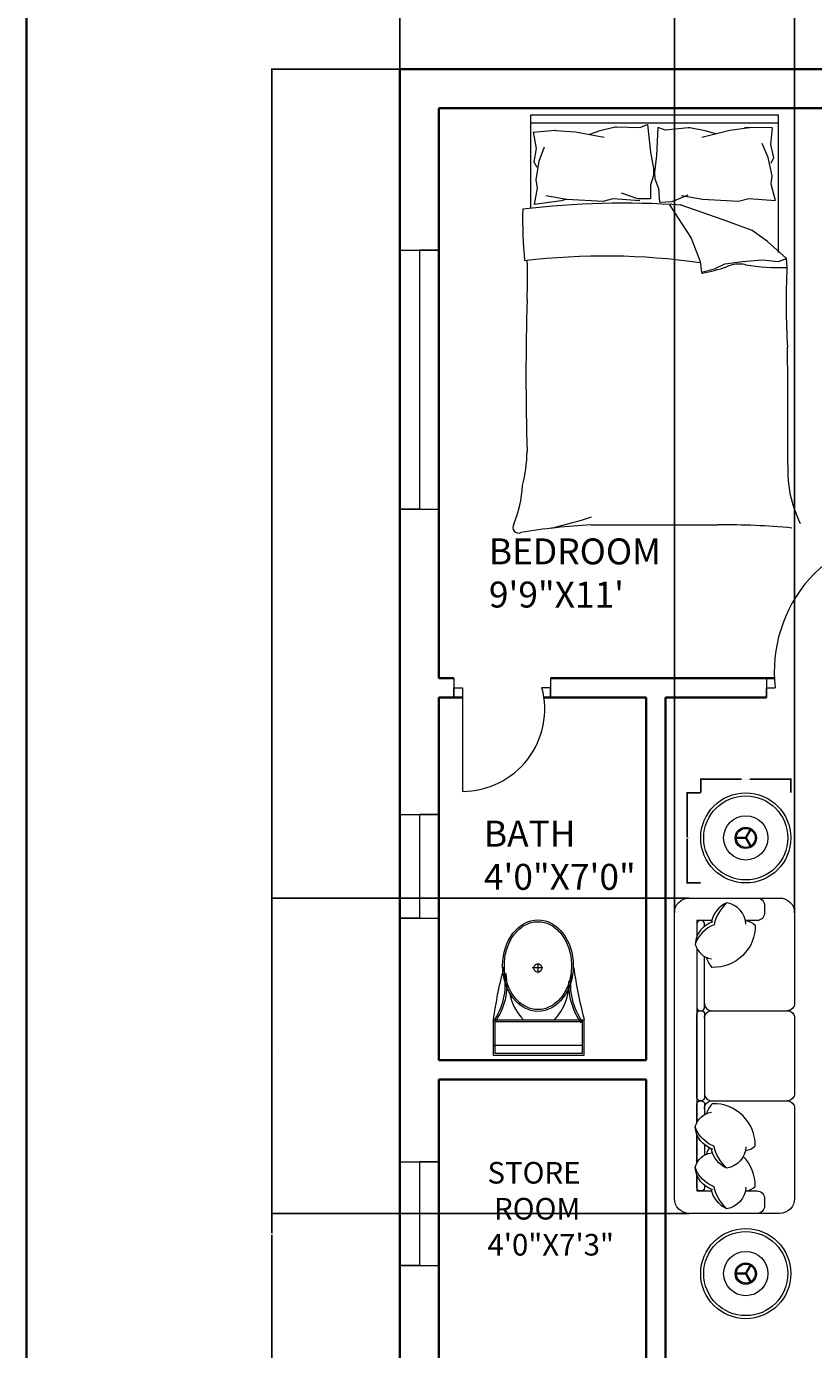
# Model space of a CAD drawing. Units: inches. Extents: x 2003 to 3241, y 1726 to 2849.
# Tile 2 of 7: x 2003 to 2186, y 2073 to 2380. Entities that reach past the tile are written whole.
import ezdxf

# ---------------------------------------------------------------- set-up
doc = ezdxf.new("R2010")
doc.units = ezdxf.units.IN
for name, color, linetype, lineweight in [('A-ANNO-DIMS', 2, 'Continuous', 18), ('A-ANNO-TTLB', 7, 'Continuous', 35), ('A-AREA-IDEN', 7, 'Continuous', 18), ('A-DOOR', 3, 'Continuous', 18), ('A-FLOR-FIXT', 9, 'Continuous', 18), ('A-FURN', 8, 'Continuous', 13), ('A-GLAZ', 4, 'Continuous', 18), ('A-WALL', 7, 'Continuous', 35)]:
    doc.layers.add(name, color=color, linetype=linetype, lineweight=lineweight)
doc.styles.get("Standard").update_dxf_attribs({"font": 'arial.ttf'})
doc.dimstyles.get("Standard").update_dxf_attribs({"dimtxt": 0.18, "dimasz": 0.18, "dimexe": 0.18, "dimexo": 0.0625, "dimgap": 0.09, "dimtad": 0, "dimtih": 1, "dimtoh": 1, "dimdec": 4, "dimzin": 0, "dimdsep": 46, "dimtxsty": 'Standard', "dimcen": 0.09, "dimadec": 0, "dimazin": 0, "dimtfac": 1, "dimtdec": 4, "dimtofl": 0, "dimtmove": 0, "dimatfit": 3, "dimfxl": 1, "dimtolj": 1, "dimtzin": 0, "dimarcsym": 0})

# ---------------------------------------------------------------- blocks, each defined once
blk = doc.blocks.new('A$C31115884')
for p, q in [((283.1, 497.7), (223.4, 497.7)), ((257.5, 466.4), (257.5, 523.2)), ((0, 200), (0, 0)), ((520, 200), (0, 200)), ((10, 190), (10, 10)), ((510, 190), (10, 190)), ((510, 10), (510, 190)), ((520, 0), (520, 200)), ((510, 54.5), (0, 54.5)), ((10, 10), (510, 10)), ((0, 0), (520, 0))]:
    blk.add_line(p, q)
blk.add_circle((255.6, 496.4), 23.6)
for centre, radius, start, end in [((2777.7, -204.6), 2807, 165.4549, 171.71327), ((-294.5, 403.3), 364.7, 324.20913, 9.34987), ((-294.5, 403.3), 374.7, 324.20913, 9.34987), ((805.8, 403.3), 364.7, 170.65013, 215.79087), ((3237, 905), 2807, 188.28673, 194.5451), ((139.5, 406.2), 293.5, 315.84364, 2.65635), ((805.8, 403.3), 374.7, 179.20365, 215.79087), ((383.6, 406.2), 293.5, 190.27735, 224.15636)]:
    blk.add_arc(centre, radius, start, end)
blk.add_ellipse((256.2, 509.9), major_axis=(0, -260.7), ratio=0.772727)
blk.add_open_spline([(256.2, 259.2), (263.1, 259.2), (270, 259.7), (287.8, 262.3), (298.7, 265.1), (319.9, 273.1), (330.2, 278.4), (350.1, 291.1), (359.7, 298.7), (377.7, 315.9), (386.2, 325.5), (401.7, 346.6), (408.8, 358.1), (421.3, 382.5), (426.8, 395.5), (435.9, 422.4), (439.5, 436.4), (444.8, 465.1), (446.5, 479.7), (447.9, 509.2), (447.6, 524), (445, 553.3), (442.7, 567.8), (436.3, 596), (432.1, 609.7), (421.9, 636), (416, 648.6), (402.5, 672.1), (395, 683), (378.6, 703), (369.8, 712.1), (351.1, 728), (341.3, 734.8), (320.9, 746.2), (310.4, 750.7), (288.9, 757.3), (278, 759.4), (256, 761), (245, 760.6), (223.1, 757.2), (212.3, 754.3), (191.1, 746.1), (180.8, 740.7), (160.9, 727.8), (151.4, 720.1), (133.5, 702.7), (125.1, 693), (109.6, 671.7), (102.6, 660.2), (90.2, 635.7), (84.9, 622.7), (76, 595.6), (72.4, 581.6), (67.2, 552.9), (65.6, 538.2), (64.4, 508.8), (64.8, 494), (67.5, 464.7), (69.9, 450.2), (76.6, 422), (80.8, 408.3), (91.1, 382.2), (97.2, 369.7), (110.8, 346.3), (118.4, 335.4), (134.8, 315.6), (143.7, 306.7), (162.4, 290.9), (172.3, 284.2), (192.8, 273), (203.3, 268.6), (224.8, 262.2), (235.8, 260.2), (249.9, 259.3), (253, 259.2), (256.2, 259.2)], degree=3, knots=[0, 0, 0, 0, 0.110105, 0.110105, 0.285049, 0.285049, 0.459994, 0.459994, 0.634938, 0.634938, 0.809882, 0.809882, 0.984827, 0.984827, 1.159771, 1.159771, 1.334715, 1.334715, 1.50966, 1.50966, 1.684604, 1.684604, 1.859549, 1.859549, 2.034493, 2.034493, 2.209437, 2.209437, 2.384382, 2.384382, 2.559326, 2.559326, 2.73427, 2.73427, 2.909215, 2.909215, 3.084159, 3.084159, 3.259103, 3.259103, 3.434048, 3.434048, 3.608992, 3.608992, 3.783936, 3.783936, 3.958881, 3.958881, 4.133825, 4.133825, 4.30877, 4.30877, 4.483714, 4.483714, 4.658658, 4.658658, 4.833603, 4.833603, 5.008547, 5.008547, 5.183491, 5.183491, 5.358436, 5.358436, 5.53338, 5.53338, 5.708324, 5.708324, 5.883269, 5.883269, 6.058213, 6.058213, 6.233158, 6.233158, 6.283185, 6.283185, 6.283185, 6.283185])
blk = doc.blocks.new('WIN-60-1')
for p, q in [((0, 60), (9, 60)), ((9, 60), (4.5, 60)), ((4.5, 60), (4.5, 0)), ((4.5, 0), (0, 0)), ((0, 0), (9, 0))]:
    blk.add_line(p, q)
blk = doc.blocks.new('WIN-24-1')
for p, q in [((0, 24), (9, 24)), ((9, 24), (4.5, 24)), ((4.5, 24), (4.5, 0)), ((4.5, 0), (0, 0)), ((0, 0), (9, 0))]:
    blk.add_line(p, q)
blk = doc.blocks.new('DOOR-BEDROOM')
for p, q in [((34.02, 2.25), (34.02, 38.25)), ((0, 4.5), (0, 0)), ((36.02, 4.5), (36.02, 0)), ((0, 0), (0, 2.25)), ((0, 2.25), (2, 2.25)), ((36.02, 2.25), (34.02, 2.25)), ((36.02, 0), (36.02, 2.25))]:
    blk.add_line(p, q)
blk.add_arc((34.02, 6.01), 32.24, 90, 186.689)
blk = doc.blocks.new('DOOR-BATH')
for p, q in [((0, 26.25), (0, 21.75)), ((22.43, 26.25), (22.43, 21.75)), ((0, 21.75), (0, 24)), ((0, 24), (2, 24)), ((2, 24), (2, 0)), ((22.43, 24), (20.43, 24)), ((22.43, 21.75), (22.43, 24))]:
    blk.add_line(p, q)
blk.add_arc((2, 19.08), 19.08, 270, 14.9552)
blk = doc.blocks.new('BED-DOUBLE')
for p, q in [((4.17, 75.16), (4.17, 96.87)), ((4.17, 96.87), (61.46, 96.87)), ((4.17, 95.03), (61.46, 95.03)), ((61.46, 96.87), (61.46, 64.97)), ((4.67, 92.87), (9.81, 93.27)), ((4.67, 92.9), (5.36, 89.08)), ((9.81, 93.27), (9.93, 93.24)), ((9.93, 93.24), (14.52, 92.9)), ((14.52, 92.9), (21.1, 91.68)), ((17.81, 92.38), (20.24, 93.24)), ((20.24, 93.24), (23.7, 94.11)), ((23.7, 94.11), (24.09, 94.11)), ((24.09, 94.11), (29.42, 93.94)), ((29.42, 93.94), (31.15, 94.63)), ((31.15, 94.63), (31.84, 88.22)), ((33.54, 93.89), (33.25, 87.44)), ((35.31, 93.3), (33.54, 93.89)), ((40.62, 93.81), (35.31, 93.3)), ((41.01, 93.83), (40.62, 93.81)), ((44.52, 93.18), (41.01, 93.83)), ((50.25, 93.19), (43.75, 91.57)), ((47, 92.47), (44.52, 93.18)), ((54.8, 93.82), (50.25, 93.19)), ((60.08, 93.81), (53.6, 93.92)), ((53.6, 93.92), (54.8, 93.82)), ((60.08, 93.81), (59.62, 89.96)), ((5.36, 89.08), (4.84, 85.96)), ((6.06, 86.14), (7.27, 89.43)), ((59.12, 86.97), (57.7, 90.18)), ((59.62, 89.96), (60.34, 86.88)), ((4.84, 85.96), (5.54, 84.75)), ((5.36, 81.8), (6.06, 86.14)), ((31.84, 88.22), (32.54, 84.4)), ((33.25, 87.44), (32.79, 83.59)), ((60.08, 82.69), (59.12, 86.97)), ((60.34, 86.88), (59.72, 85.62)), ((32.54, 82.84), (31.84, 80.59)), ((32.54, 84.4), (32.54, 82.84)), ((32.79, 83.59), (32.89, 82.03)), ((5.02, 76.08), (5.71, 79.9)), ((5.71, 79.9), (5.36, 81.8)), ((31.84, 80.59), (31.84, 77.38)), ((32.89, 82.03), (33.72, 79.83)), ((33.72, 79.83), (33.93, 76.62)), ((59.85, 80.77), (60.08, 82.69)), ((60.78, 77), (59.85, 80.77)), ((11.13, 76.95), (5.02, 76.08)), ((7.65, 78.14), (12.48, 77.34)), ((12.48, 77.34), (11.13, 76.95)), ((12.48, 77.34), (20.89, 76.82)), ((20.89, 76.82), (23.24, 77.49)), ((23.24, 77.49), (29.39, 77)), ((28.9, 77.38), (25.13, 78.68)), ((31.84, 77.38), (28.9, 77.38)), ((33.93, 76.62), (36.87, 76.8)), ((36.87, 76.8), (40.55, 78.34)), ((39.04, 78.14), (43.87, 77.34)), ((43.87, 77.34), (52.28, 76.82)), ((52.28, 76.82), (54.63, 77.49)), ((54.63, 77.49), (60.78, 77)), ((36.28, 76.03), (41.3, 68.25)), ((48.73, 72.52), (38.73, 76.03)), ((55.41, 70.1), (48.73, 72.52)), ((41.3, 68.25), (43.34, 62.87)), ((58.94, 67.51), (55.41, 70.1)), ((63.38, 63.61), (58.94, 67.51)), ((43.34, 62.87), (43.71, 60.45)), ((46.68, 61.2), (49.1, 62.31)), ((49.1, 62.31), (53.18, 62.87)), ((53.18, 62.87), (57.82, 63.24)), ((57.82, 63.24), (61.54, 62.87)), ((61.54, 62.87), (63.38, 63.61)), ((63.48, 61.52), (63.38, 63.61, 4.64)), ((43.71, 60.45), (46.68, 61.2)), ((18.06, 1.87), (47.57, 1.87))]:
    blk.add_line(p, q)
for centre, radius, start, end in [((102.1, 72.78), 99.87, 178.7218, 185.604), ((25.61, -121.38), 197.77, 86.0865, 96.7821), ((21.29, -90.53), 154.68, 81.7845, 96.9006), ((-200.58, 59.5), 203.94, 358.4762, 1.0082), ((37.35, 95.1), 35.55, 280.6617, 289.8806), ((52.44, 54.83), 7.46, 78.6608, 113.7384), ((61.53, 104.85), 43.38, 259.8763, 272.5657), ((218.51, 53.34), 155.25, 176.9791, 183.8365), ((43.92, 60.38), 0.221, 160.2464, 271.1377), ((581.23, 36.19), 578.22, 178.22771, 181.71854), ((-5405.34, 15.56), 5469.02, 0.00217, 0.28689), ((-32.25, 19.53), 35.53, 346.0648, 358.9113), ((91.3, 14.55), 27.65, 177.4714, 206.4681), ((-25.97, 12.62), 28.25, 337.9751, 356.652), ((-20.65, 125.3), 127.63, 283.3832, 287.7053), ((1.3, 1.3), 1.31, 146.1736, 293.4781), ((25.69, -143.9), 145.97, 92.9958, 99.4091), ((49.34, -157.62), 159.5, 84.4998, 90.6351)]:
    blk.add_arc(centre, radius, start, end)
blk = doc.blocks.new('TABLE-ROUND')
at = {"ltscale": 0.03}
for p, q in [((10.34, 10.49), (11.57, 12.62)), ((10.53, 10.38), (11.76, 12.51)), ((10.44, 10.55), (7.99, 10.55)), ((10.44, 10.33), (7.99, 10.33)), ((10.34, 10.38), (11.57, 8.26)), ((10.53, 10.49), (11.76, 8.37))]:
    blk.add_line(p, q, dxfattribs=at)
for radius in [10.44, 5.13, 2.46, 2.2]:
    blk.add_circle((10.44, 10.44), radius, dxfattribs=at)
blk.add_circle((10.44, 10.44), 9.74)
blk = doc.blocks.new('*D60')
at = {"layer": 'A-ANNO-DIMS', "color": 0, "lineweight": -2, "transparency": 16777216}
for p, q in [((2159.44, 2202.38), (2159.44, 2205.63)), ((2159.62, 2205.45), (2168.92, 2205.45)), ((2180.14, 2205.45), (2170.85, 2205.45)), ((2180.32, 2202.38), (2180.32, 2205.63))]:
    blk.add_line(p, q, dxfattribs=at)
at = {"layer": 'A-ANNO-DIMS', "color": 0, "transparency": 16777216}
for points in [[(2159.62, 2205.48), (2159.62, 2205.42), (2159.44, 2205.45)], [(2180.14, 2205.48), (2180.14, 2205.42), (2180.32, 2205.45)]]:
    blk.add_solid(points, dxfattribs=at)
at = {"layer": 'Defpoints', "color": 0, "transparency": 16777216}
for p in [(2180.32, 2205.45), (2159.44, 2202.32), (2180.32, 2202.32)]:
    blk.add_point(p, dxfattribs=at)
at = {"layer": 'A-ANNO-DIMS', "color": 0, "transparency": 16777216, "insert": (2169.88, 2205.45), "char_height": 0.18, "attachment_point": 5}
blk.add_mtext('\\A1;TABLE 21 TYP.', dxfattribs=at)
blk = doc.blocks.new('*D61')
at = {"layer": 'A-ANNO-DIMS', "color": 0, "lineweight": -2, "transparency": 16777216}
for p, q in [((2159.38, 2202.32), (2156.13, 2202.32)), ((2156.31, 2202.14), (2156.31, 2192.06)), ((2156.31, 2181.62), (2156.31, 2191.7)), ((2159.38, 2181.44), (2156.13, 2181.44))]:
    blk.add_line(p, q, dxfattribs=at)
at = {"layer": 'A-ANNO-DIMS', "color": 0, "transparency": 16777216}
for points in [[(2156.28, 2202.14), (2156.34, 2202.14), (2156.31, 2202.32)], [(2156.28, 2181.62), (2156.34, 2181.62), (2156.31, 2181.44)]]:
    blk.add_solid(points, dxfattribs=at)
at = {"layer": 'Defpoints', "color": 0, "transparency": 16777216}
for p in [(2156.31, 2202.32), (2159.44, 2202.32), (2159.44, 2181.44)]:
    blk.add_point(p, dxfattribs=at)
at = {"layer": 'A-ANNO-DIMS', "color": 0, "transparency": 16777216, "insert": (2156.31, 2191.88), "char_height": 0.18, "attachment_point": 5}
blk.add_mtext('\\A1;21 TYP.', dxfattribs=at)
blk = doc.blocks.new('*D64')
at = {"layer": 'A-ANNO-DIMS', "color": 0, "lineweight": -2, "transparency": 16777216}
for p, q in [((2089.78, 2369.98), (2089.78, 2399.74)), ((2089.96, 2399.56), (2197.49, 2399.56)), ((2305.6, 2399.56), (2198.07, 2399.56)), ((2305.78, 2369.98), (2305.78, 2399.74))]:
    blk.add_line(p, q, dxfattribs=at)
at = {"layer": 'A-ANNO-DIMS', "color": 0, "transparency": 16777216}
for points in [[(2089.96, 2399.59), (2089.96, 2399.53), (2089.78, 2399.56)], [(2305.6, 2399.59), (2305.6, 2399.53), (2305.78, 2399.56)]]:
    blk.add_solid(points, dxfattribs=at)
at = {"layer": 'Defpoints', "color": 0, "transparency": 16777216}
for p in [(2305.78, 2399.56), (2089.78, 2369.91), (2305.78, 2369.91)]:
    blk.add_point(p, dxfattribs=at)
at = {"layer": 'A-ANNO-DIMS', "color": 0, "transparency": 16777216, "insert": (2197.78, 2399.56), "char_height": 0.18, "attachment_point": 5}
blk.add_mtext('\\A1;216', dxfattribs=at)
blk = doc.blocks.new('*D65')
at = {"layer": 'A-ANNO-DIMS', "color": 0, "lineweight": -2, "transparency": 16777216}
for p, q in [((2089.72, 2369.91), (2059.95, 2369.91)), ((2060.13, 2369.73), (2060.13, 2100.35)), ((2060.13, 1830.59), (2060.13, 2099.98)), ((2089.72, 1830.41), (2059.95, 1830.41))]:
    blk.add_line(p, q, dxfattribs=at)
at = {"layer": 'A-ANNO-DIMS', "color": 0, "transparency": 16777216}
for points in [[(2060.1, 2369.73), (2060.16, 2369.73), (2060.13, 2369.91)], [(2060.1, 1830.59), (2060.16, 1830.59), (2060.13, 1830.41)]]:
    blk.add_solid(points, dxfattribs=at)
at = {"layer": 'Defpoints', "color": 0, "transparency": 16777216}
for p in [(2060.13, 2369.91), (2089.78, 2369.91), (2089.78, 1830.41)]:
    blk.add_point(p, dxfattribs=at)
at = {"layer": 'A-ANNO-DIMS', "color": 0, "transparency": 16777216, "insert": (2060.13, 2100.16), "char_height": 0.18, "attachment_point": 5}
blk.add_mtext('\\A1;539.5', dxfattribs=at)
blk = doc.blocks.new('*D68')
at = {"layer": 'A-ANNO-DIMS', "color": 0, "lineweight": -2, "transparency": 16777216}
for p, q in [((2153.35, 2174.54), (2153.35, 2399.74)), ((2153.53, 2399.56), (2166.88, 2399.56)), ((2181.01, 2399.56), (2167.67, 2399.56)), ((2181.19, 2174.54), (2181.19, 2399.74))]:
    blk.add_line(p, q, dxfattribs=at)
at = {"layer": 'A-ANNO-DIMS', "color": 0, "transparency": 16777216}
for points in [[(2153.53, 2399.59), (2153.53, 2399.53), (2153.35, 2399.56)], [(2181.01, 2399.59), (2181.01, 2399.53), (2181.19, 2399.56)]]:
    blk.add_solid(points, dxfattribs=at)
at = {"layer": 'Defpoints', "color": 0, "transparency": 16777216}
for p in [(2181.19, 2399.56), (2153.35, 2174.48), (2181.19, 2174.48)]:
    blk.add_point(p, dxfattribs=at)
at = {"layer": 'A-ANNO-DIMS', "color": 0, "transparency": 16777216, "insert": (2167.27, 2399.56), "char_height": 0.18, "attachment_point": 5}
blk.add_mtext('\\A1;27.84', dxfattribs=at)
blk = doc.blocks.new('*D69')
at = {"layer": 'A-ANNO-DIMS', "color": 0, "lineweight": -2, "transparency": 16777216}
for p, q in [((2156.77, 2177.96), (2059.95, 2177.96)), ((2060.13, 2177.78), (2060.13, 2141.61)), ((2060.13, 2105.07), (2060.13, 2141.24)), ((2156.77, 2104.89), (2059.95, 2104.89))]:
    blk.add_line(p, q, dxfattribs=at)
at = {"layer": 'A-ANNO-DIMS', "color": 0, "transparency": 16777216}
for points in [[(2060.1, 2177.78), (2060.16, 2177.78), (2060.13, 2177.96)], [(2060.1, 2105.07), (2060.16, 2105.07), (2060.13, 2104.89)]]:
    blk.add_solid(points, dxfattribs=at)
at = {"layer": 'Defpoints', "color": 0, "transparency": 16777216}
for p in [(2060.13, 2177.96), (2156.83, 2177.96), (2156.83, 2104.89)]:
    blk.add_point(p, dxfattribs=at)
at = {"layer": 'A-ANNO-DIMS', "color": 0, "transparency": 16777216, "insert": (2060.13, 2141.42), "char_height": 0.18, "attachment_point": 5}
blk.add_mtext('\\A1;73.07', dxfattribs=at)

msp = doc.modelspace()

# ---------------------------------------------------------------- linework, layer by layer
at = {"layer": 'A-ANNO-TTLB'}
msp.add_lwpolyline([(2003.2633, 2848.7261), (3241.1194, 2848.7261), (3241.1194, 1726.227), (2003.2633, 1726.227)], close=True, dxfattribs=at)
at = {"layer": 'A-FURN', "ltscale": 0.03}
msp.add_lwpolyline([(2177.7119, 2177.9617, -0.41421356), (2181.1916, 2174.4819), (2181.1916, 2153.6036, -0.41421356), (2179.4517, 2151.8637, -0.41421356), (2181.1916, 2150.1239), (2181.1916, 2132.7252, -0.41421356), (2179.4517, 2130.9854, -0.41421356), (2181.1916, 2129.2455), (2181.1916, 2108.3672, -0.41421356), (2177.7119, 2104.8874), (2156.8335, 2104.8874, -0.41421356), (2153.3538, 2108.3672), (2153.3538, 2174.4819, -0.41421356), (2156.8335, 2177.9617)], format="xyb", close=True, dxfattribs=at)
at = {"layer": 'A-FURN'}
for points in [[(2165.5164, 2176.8544, 0.14772988), (2162.5263, 2171.7692, 0.21334276), (2158.1407, 2167.2824, 0.17866181)], [(2169.9019, 2171.8689, 0.35677236), (2165.5164, 2176.8544, 0.24954205), (2161.9023, 2172.3371, -9.61688035)], [(2172.4923, 2177.9617, -0.41421356), (2174.2322, 2176.2218), (2174.2322, 2174.4819, -0.41421356), (2172.4923, 2172.7421), (2169.7966, 2172.7421)], [(2160.3133, 2171.4144), (2160.3133, 2172.0461, 0.41421356), (2159.6173, 2172.7421), (2159.2693, 2172.7421, 0.41421356), (2158.5734, 2172.0461)], [(2169.7958, 2172.7459, -0.16554063), (2172.0947, 2171.6695, -0.42598917), (2162.1276, 2161.8981, -0.12152332), (2160.7538, 2164.2177, 7.11546429)], [(2162.288, 2172.4718, 0.30666349), (2158.1407, 2167.2824, 0.30632997), (2161.9282, 2163.8923, -0.87284716)], [(2158.5734, 2172.0461), (2158.5734, 2169.0819, 0.41421356)], [(2158.5734, 2166.1874), (2158.5734, 2152.5597, 0.41421356), (2159.2693, 2151.8637), (2159.6173, 2151.8637, 0.41421356), (2160.3133, 2152.5597), (2160.3133, 2164.4355, 0.41421356)], [(2160.3133, 2153.6036, 0.41421356), (2162.0531, 2151.8637), (2179.4517, 2151.8637, 0.41421356)], [(2160.3133, 2150.1239, -0.41421356), (2162.0531, 2151.8637)], [(2158.5734, 2126.0343), (2158.5734, 2130.2894, -0.41421356), (2159.2693, 2130.9854), (2159.6173, 2130.9854, -0.41421356), (2160.3133, 2130.2894), (2160.3133, 2127.7862, -0.41421356)], [(2160.3133, 2132.7252, 0.41421356), (2162.0531, 2130.9854)], [(2160.3133, 2129.2455, -0.41421356), (2162.0531, 2130.9854), (2179.4517, 2130.9854, -0.41421356)], [(2169.7958, 2119.4758, 0.16554063), (2172.0947, 2120.5521, 0.42598917), (2162.1276, 2130.3235, 0.12152332), (2160.7538, 2128.004, -7.11546429)], [(2162.288, 2119.7499, -0.30666349), (2158.1407, 2124.9393, -0.30632997), (2161.9282, 2128.3294, 0.87284716)], [(2165.5164, 2115.3673, -0.14772988), (2162.5263, 2120.4524, -0.21334276), (2158.1407, 2124.9393, -0.17866181)], [(2158.5734, 2116.6617), (2158.5734, 2123.1398, -0.41421356)], [(2160.3133, 2120.8073), (2160.3133, 2118.4136, -0.41421356)], [(2162.288, 2110.3773, -0.30666349), (2158.1407, 2115.5667, -0.30632997), (2161.9282, 2118.9568, 0.87284716)], [(2161.434, 2120.0901, 0.07186538), (2160.7538, 2118.6314, -7.11546429)], [(2169.9019, 2120.3527, -0.35677236), (2165.5164, 2115.3673, -0.24954205), (2161.9023, 2119.8846, 9.61688035)], [(2169.7958, 2110.1032, 0.16554063), (2172.0947, 2111.1796, 0.20023115), (2169.2949, 2118.0862, 0.12152332)], [(2165.5164, 2105.9947, -0.14772988), (2162.5263, 2111.0799, -0.21334276), (2158.1407, 2115.5667, -0.17866181)], [(2158.5734, 2113.7672), (2158.5734, 2110.107), (2161.9926, 2110.107, -0.41421356)], [(2158.5734, 2110.803), (2158.5734, 2113.7672, -0.41421356)], [(2160.3133, 2111.4347), (2160.3133, 2110.803, -0.41421356), (2159.6173, 2110.107), (2159.2693, 2110.107, -0.41421356), (2158.5734, 2110.803)], [(2169.9019, 2110.9802, -0.35677236), (2165.5164, 2105.9947, -0.24954205), (2161.9023, 2110.512, 9.61688035)], [(2169.7966, 2110.107), (2172.4923, 2110.107, -0.41421356), (2174.2322, 2108.3672), (2174.2322, 2106.6273, -0.41421356), (2172.4923, 2104.8874)]]:
    msp.add_lwpolyline(points, format="xyb", dxfattribs=at)
for points in [[(2161.9926, 2172.7421), (2158.5734, 2172.7421), (2158.5734, 2169.0819)], [(2158.5734, 2166.1874), (2158.5734, 2126.0343)], [(2158.5734, 2123.1398), (2158.5734, 2116.6617)]]:
    msp.add_lwpolyline(points, dxfattribs=at)
msp.add_lwpolyline([(2158.5734, 2131.6813), (2158.5734, 2151.1678, -0.41421356), (2159.2693, 2151.8637), (2159.6173, 2151.8637, -0.41421356), (2160.3133, 2151.1678), (2160.3133, 2131.6813, -0.41421356), (2159.6173, 2130.9854), (2159.2693, 2130.9854, -0.41421356)], format="xyb", close=True, dxfattribs=at)
at = {"layer": 'A-WALL'}
for p, q in [((2089.7784, 2369.9135), (2305.7784, 2369.9135)), ((2089.7784, 2369.9135), (2305.7784, 2369.9135)), ((2089.7784, 2369.9135), (2089.7784, 1830.4135)), ((2098.7784, 2360.9135), (2215.7784, 2360.9135)), ((2098.7784, 2360.9135), (2098.7784, 2228.9135)), ((2098.7784, 2228.9135), (2102.2463, 2228.9135)), ((2124.6771, 2228.9135), (2176.5139, 2228.9135)), ((2098.7784, 2224.4135), (2104.2463, 2224.4135)), ((2098.7784, 2224.4135), (2098.7784, 2140.4135)), ((2123.135, 2224.4135), (2146.7784, 2224.4135)), ((2146.7784, 2224.4135), (2146.7784, 2140.4135)), ((2151.2784, 2224.4135), (2151.2784, 2048.9135)), ((2151.2784, 2224.4135), (2174.6982, 2224.4135)), ((2098.7784, 2140.4135), (2146.7784, 2140.4135)), ((2098.7784, 2135.9135), (2146.7784, 2135.9135)), ((2098.7784, 2135.9135), (2098.7784, 2048.9135)), ((2146.7784, 2135.9135), (2146.7784, 2048.9135))]:
    msp.add_line(p, q, dxfattribs=at)

# ---------------------------------------------------------------- block references
at = {"layer": 'A-DOOR'}
for name, p in [('DOOR-BEDROOM', (2174.698, 2224.414)), ('DOOR-BATH', (2102.246, 2202.664))]:
    msp.add_blockref(name, p, dxfattribs=at)
at = {"layer": 'A-FLOR-FIXT', "xscale": 0.0406268506401408, "yscale": 0.0406268506401408, "zscale": 0.0406268506401408}
msp.add_blockref('A$C31115884', (2111.336, 2141.5799), dxfattribs=at)
at = {"layer": 'A-FURN'}
for name, p in [('BED-DOUBLE', (2115.953, 2262.5)), ('TABLE-ROUND', (2159.443, 2181.441))]:
    msp.add_blockref(name, p, dxfattribs=at)
at = {"layer": 'A-FURN', "rotation": 239.9999999970011}
msp.add_blockref('TABLE-ROUND', (2166.0613, 2105.2292), dxfattribs=at)
at = {"layer": 'A-GLAZ'}
for name, p in [('WIN-60-1', (2089.778, 2268.0124)), ('WIN-24-1', (2089.778, 2173.279)), ('WIN-24-1', (2089.778, 2092.8237))]:
    msp.add_blockref(name, p, dxfattribs=at)

# ---------------------------------------------------------------- texts
at = {"layer": 'A-AREA-IDEN', "attachment_point": 1}
for s, width, insert, char_height in [('BEDROOM\\P9\'9"X11\'', 61.126503, (2110.3817, 2261.243), 6), ('BATH\\P4\'0"X7\'0"', 56.046697, (2109.2241, 2195.8629), 6), ('STORE\\P ROOM\\P4\'0"X7\'3"', 54.193419, (2110.0436, 2116.8234), 5)]:
    msp.add_mtext_dynamic_manual_height_columns(s, width=width, gutter_width=12.5, heights=[0], dxfattribs=dict(at, insert=insert, char_height=char_height))

# ---------------------------------------------------------------- dimensions: what is measured, and where the dimension line sits
at = {"layer": 'A-ANNO-DIMS'}
for base, p1, p2, override, picture, middle in [((2305.7784, 2399.5635), (2089.7784, 2369.9135), (2305.7784, 2369.9135), {"dimdec": 0, "dimlfac": 1, "dimrnd": 0, "dimzin": 0, "dimdsep": 46, "dimlunit": 2}, '*D64', (2197.7784, 2399.5635)), ((2181.1916, 2399.5635), (2153.3538, 2174.4819), (2181.1916, 2174.4819), {"dimdec": 2, "dimlfac": 1, "dimrnd": 0, "dimzin": 0, "dimdsep": 46, "dimlunit": 2}, '*D68', (2167.2727, 2399.5635))]:
    dim = msp.add_linear_dim(base=base, p1=p1, p2=p2, dimstyle='Standard', override=override, dxfattribs=at)
    dim.commit()
    dim.dimension.update_dxf_attribs({"geometry": picture, "text_midpoint": middle})
for base, p1, p2, override, picture, middle in [((2060.1284, 2369.9135), (2089.7784, 1830.4135), (2089.7784, 2369.9135), {"dimdec": 1, "dimlfac": 1, "dimrnd": 0, "dimzin": 0, "dimdsep": 46, "dimlunit": 2}, '*D65', (2060.1284, 2100.1635)), ((2060.1284, 2177.9617), (2156.8335, 2104.8874), (2156.8335, 2177.9617), {"dimdec": 2, "dimlfac": 1, "dimrnd": 0, "dimzin": 0, "dimdsep": 46, "dimlunit": 2}, '*D69', (2060.1284, 2141.4246))]:
    dim = msp.add_linear_dim(base=base, p1=p1, p2=p2, angle=90, dimstyle='Standard', override=override, dxfattribs=at)
    dim.commit()
    dim.dimension.update_dxf_attribs({"geometry": picture, "text_midpoint": middle})
dim = msp.add_linear_dim(base=(2180.3217, 2205.4515), p1=(2159.4433, 2202.3197), p2=(2180.3217, 2202.3197), text='TABLE <> TYP.', dimstyle='Standard', override={"dimdec": 0, "dimlfac": 1, "dimrnd": 0, "dimzin": 0, "dimdsep": 46, "dimlunit": 2}, dxfattribs=at)
dim.commit()
dim.dimension.update_dxf_attribs({"geometry": '*D60', "text_midpoint": (2169.8825, 2205.4515)})
dim = msp.add_linear_dim(base=(2156.3116, 2202.3197), p1=(2159.4433, 2181.4414), p2=(2159.4433, 2202.3197), angle=90, text='<> TYP.', dimstyle='Standard', override={"dimdec": 0, "dimlfac": 1, "dimrnd": 0, "dimzin": 0, "dimdsep": 46, "dimlunit": 2}, dxfattribs=at)
dim.commit()
dim.dimension.update_dxf_attribs({"geometry": '*D61', "text_midpoint": (2156.3116, 2191.8806)})

doc.saveas('drawing.dxf')
